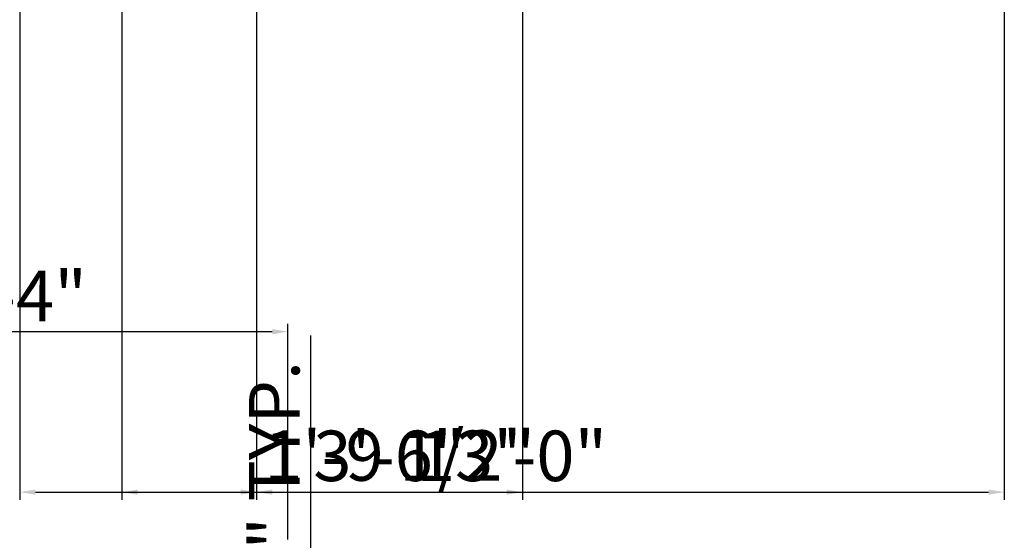
# Model space of a CAD drawing. Units: inches. Extents: x 2257 to 3678, y 834 to 1975.
# Tile 11 of 16: x 3338 to 3494, y 1594 to 1677. Entities that reach past the tile are written whole.
import ezdxf

# ---------------------------------------------------------------- set-up
doc = ezdxf.new("R2010")
doc.units = ezdxf.units.IN
doc.layers.add('A-ANNO-DIMS', color=2, linetype='Continuous', lineweight=18)
doc.styles.get("Standard").update_dxf_attribs({"font": 'arial.ttf'})
doc.dimstyles.new('ISO-25', dxfattribs={"dimtxt": 8, "dimasz": 2.5, "dimexe": 1.25, "dimexo": 0.625, "dimtad": 1, "dimdec": 0, "dimlunit": 3, "dimtxsty": 'Standard', "dimcen": 2.5, "dimadec": 0, "dimazin": 0, "dimtfac": 1, "dimtdec": 0, "dimtmove": 0, "dimatfit": 3, "dimfxl": 1, "dimarcsym": 0})

# ---------------------------------------------------------------- blocks, each defined once
blk = doc.blocks.new('*D70')
at = {"layer": 'A-ANNO-DIMS', "color": 0, "lineweight": -2, "transparency": 16777216}
for p, q in [((3383.84, 1485.58), (3383.84, 1626.53)), ((3377.72, 1485.58), (3385.09, 1485.58)), ((3383.84, 1443.08), (3383.84, 1483.08)), ((3377.72, 1440.58), (3385.09, 1440.58))]:
    blk.add_line(p, q, dxfattribs=at)
at = {"layer": 'A-ANNO-DIMS', "color": 0, "transparency": 16777216}
for points in [[(3383.42, 1483.08), (3384.26, 1483.08), (3383.84, 1485.58)], [(3383.42, 1443.08), (3384.26, 1443.08), (3383.84, 1440.58)]]:
    blk.add_solid(points, dxfattribs=at)
at = {"layer": 'Defpoints', "color": 0, "transparency": 16777216}
for p in [(3377.09, 1485.58), (3383.84, 1485.58), (3377.09, 1440.58)]:
    blk.add_point(p, dxfattribs=at)
at = {"layer": 'A-ANNO-DIMS', "color": 0, "transparency": 16777216, "insert": (3379.07, 1557.3), "char_height": 8, "attachment_point": 5, "rotation": 90}
blk.add_mtext('KITCHEN DOOR 3\'-9" TYP.', dxfattribs=at)
blk = doc.blocks.new('*D110')
at = {"layer": 'A-ANNO-DIMS', "color": 0, "lineweight": -2, "transparency": 16777216}
for p, q in [((3292.39, 1594.2), (3292.39, 1628.38)), ((3294.89, 1627.13), (3377.71, 1627.13)), ((3380.21, 1594.2), (3380.21, 1628.38))]:
    blk.add_line(p, q, dxfattribs=at)
at = {"layer": 'A-ANNO-DIMS', "color": 0, "transparency": 16777216}
for points in [[(3294.89, 1627.54), (3294.89, 1626.71), (3292.39, 1627.13)], [(3377.71, 1627.54), (3377.71, 1626.71), (3380.21, 1627.13)]]:
    blk.add_solid(points, dxfattribs=at)
at = {"layer": 'Defpoints', "color": 0, "transparency": 16777216}
for p in [(3380.21, 1627.13), (3292.39, 1593.58), (3380.21, 1593.58)]:
    blk.add_point(p, dxfattribs=at)
at = {"layer": 'A-ANNO-DIMS', "color": 0, "transparency": 16777216, "insert": (3336.3, 1631.75), "char_height": 8, "attachment_point": 5}
blk.add_mtext('7\'-4"', dxfattribs=at)
blk = doc.blocks.new('*D137')
at = {"layer": 'A-ANNO-DIMS', "color": 0, "lineweight": -2, "transparency": 16777216}
for p, q in [((3337.7, 1696.22), (3337.7, 1600.44)), ((3493.7, 1696.22), (3493.7, 1600.44)), ((3340.2, 1601.69), (3491.2, 1601.69))]:
    blk.add_line(p, q, dxfattribs=at)
at = {"layer": 'A-ANNO-DIMS', "color": 0, "transparency": 16777216}
for points in [[(3340.2, 1602.1), (3340.2, 1601.27), (3337.7, 1601.69)], [(3491.2, 1602.1), (3491.2, 1601.27), (3493.7, 1601.69)]]:
    blk.add_solid(points, dxfattribs=at)
at = {"layer": 'Defpoints', "color": 0, "transparency": 16777216}
for p in [(3337.7, 1696.84), (3493.7, 1696.84), (3493.7, 1601.69)]:
    blk.add_point(p, dxfattribs=at)
at = {"layer": 'A-ANNO-DIMS', "color": 0, "transparency": 16777216, "insert": (3415.7, 1606.4), "char_height": 8, "attachment_point": 5}
blk.add_mtext('13\'-0"', dxfattribs=at)
blk = doc.blocks.new('*D143')
at = {"layer": 'A-ANNO-DIMS', "color": 0, "lineweight": -2, "transparency": 16777216}
for p, q in [((3353.91, 1804.83), (3353.91, 1600.44)), ((3375.21, 1803.92), (3375.21, 1600.44)), ((3356.41, 1601.69), (3372.71, 1601.69)), ((3375.21, 1601.69), (3418.11, 1601.69))]:
    blk.add_line(p, q, dxfattribs=at)
at = {"layer": 'A-ANNO-DIMS', "color": 0, "transparency": 16777216}
for points in [[(3356.41, 1602.1), (3356.41, 1601.27), (3353.91, 1601.69)], [(3372.71, 1602.1), (3372.71, 1601.27), (3375.21, 1601.69)]]:
    blk.add_solid(points, dxfattribs=at)
at = {"layer": 'Defpoints', "color": 0, "transparency": 16777216}
for p in [(3353.91, 1805.46), (3375.21, 1804.55), (3375.21, 1601.69)]:
    blk.add_point(p, dxfattribs=at)
at = {"layer": 'A-ANNO-DIMS', "color": 0, "transparency": 16777216, "insert": (3397.91, 1606.45), "char_height": 8, "attachment_point": 5}
blk.add_mtext('1\'-9 1/2"', dxfattribs=at)
blk = doc.blocks.new('*D144')
at = {"layer": 'A-ANNO-DIMS', "color": 0, "lineweight": -2, "transparency": 16777216}
for p, q in [((3375.21, 1803.92), (3375.21, 1600.44)), ((3417.35, 1803.92), (3417.35, 1600.44)), ((3377.71, 1601.69), (3414.85, 1601.69))]:
    blk.add_line(p, q, dxfattribs=at)
at = {"layer": 'A-ANNO-DIMS', "color": 0, "transparency": 16777216}
for points in [[(3377.71, 1602.1), (3377.71, 1601.27), (3375.21, 1601.69)], [(3414.85, 1602.1), (3414.85, 1601.27), (3417.35, 1601.69)]]:
    blk.add_solid(points, dxfattribs=at)
at = {"layer": 'Defpoints', "color": 0, "transparency": 16777216}
for p in [(3375.21, 1804.55), (3417.35, 1804.55), (3417.35, 1601.69)]:
    blk.add_point(p, dxfattribs=at)
at = {"layer": 'A-ANNO-DIMS', "color": 0, "transparency": 16777216, "insert": (3396.28, 1606.4), "char_height": 8, "attachment_point": 5}
blk.add_mtext('3\'-6"', dxfattribs=at)

msp = doc.modelspace()

# ---------------------------------------------------------------- dimensions: what is measured, and where the dimension line sits
at = {"layer": 'A-ANNO-DIMS'}
for base, p1, p2, picture, middle in [((3375.21, 1601.69), (3353.91, 1805.46), (3375.21, 1804.55), '*D143', (3397.91, 1606.45)), ((3417.35, 1601.69), (3375.21, 1804.55), (3417.35, 1804.55), '*D144', (3396.28, 1606.4)), ((3493.7, 1601.69), (3337.7, 1696.84), (3493.7, 1696.84), '*D137', (3415.7, 1606.4)), ((3380.21, 1627.13), (3292.39, 1593.58), (3380.21, 1593.58), '*D110', (3336.3, 1631.75))]:
    dim = msp.add_linear_dim(base=base, p1=p1, p2=p2, dimstyle='ISO-25', override={"dimdec": 1, "dimlfac": 1, "dimrnd": 0, "dimzin": 1, "dimdsep": 46, "dimlunit": 4, "dimfrac": 2}, dxfattribs=at)
    dim.commit()
    dim.dimension.update_dxf_attribs({"geometry": picture, "text_midpoint": middle})
dim = msp.add_linear_dim(base=(3383.84, 1485.58), p1=(3377.09, 1440.58), p2=(3377.09, 1485.58), angle=90, text='KITCHEN DOOR <> TYP.', dimstyle='ISO-25', override={"dimdec": 1, "dimlfac": 1, "dimrnd": 0, "dimzin": 1, "dimdsep": 46, "dimlunit": 4, "dimfrac": 2}, dxfattribs=at)
dim.commit()
dim.dimension.update_dxf_attribs({"geometry": '*D70', "text_midpoint": (3379.07, 1557.3)})

doc.saveas('drawing.dxf')
